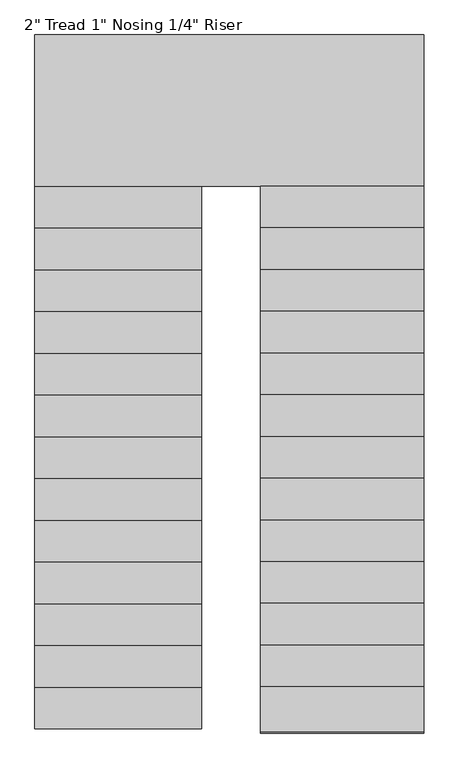
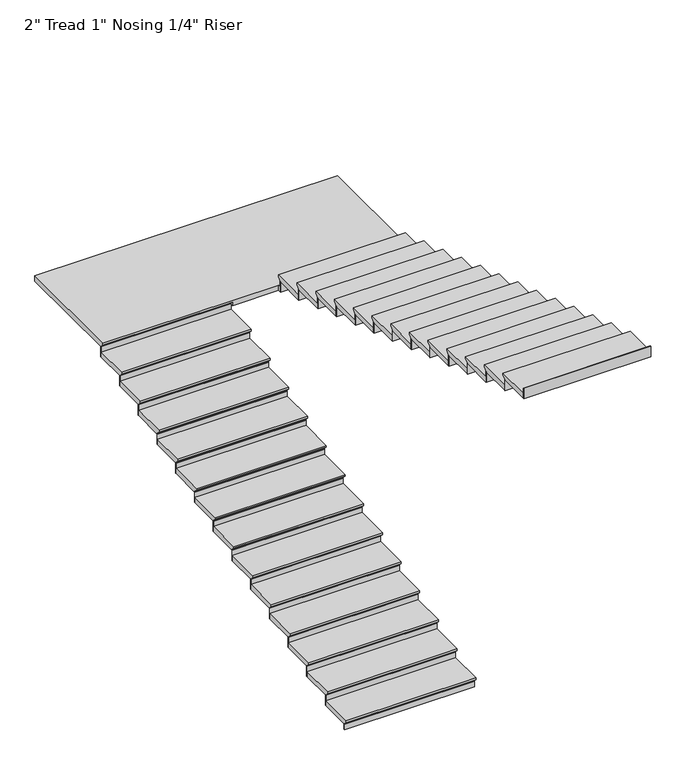
"""IFC4 building model written with IfcOpenShell, lengths in millimetres: stair flight geometry."""

from ifc_helpers import new_model, si_unit, origin, place, context, project, spatial, faceted_brep, source, transform, mapped, element, save


def stair_flight_ccf7fef2(model_context):
    return source(origin(), model_context, "Body", "Brep", [
        faceted_brep([(-629.5987998, 2564.5067329, 12885.9642857), (-629.5987998, 2564.5067329, 12905.0142857), (-1848.7987998, 2564.5067329, 12905.0142857), (-1848.7987998, 2564.5067329, 12885.9642857), (-629.5987998, 2589.9067329, 12860.5642857), (-1848.7987998, 2589.9067329, 12860.5642857), (-629.5987998, 2894.7067329, 12905.0142857), (-1848.7987998, 2894.7067329, 12905.0142857), (-1848.7987998, 2589.9067329, 12854.2142857), (-1848.7987998, 2894.7067329, 12854.2142857), (-629.5987998, 2894.7067329, 12854.2142857), (-629.5987998, 2589.9067329, 12854.2142857)], [[[0, 1, 2, 3]], [[4, 0, 3, 5]], [[2, 1, 6, 7]], [[8, 9, 10, 11]], [[2, 7, 9, 8, 5, 3]], [[8, 11, 4, 5]], [[6, 1, 0, 4, 11, 10]], [[7, 6, 10, 9]]]),
        faceted_brep([(-629.5987998, 2589.9067329, 12854.2142857), (-629.5987998, 2589.9067329, 12801.6), (-629.5987998, 2596.2567329, 12801.6), (-629.5987998, 2596.2567329, 12854.2142857), (-1848.7987998, 2589.9067329, 12854.2142857), (-1848.7987998, 2596.2567329, 12854.2142857), (-1848.7987998, 2596.2567329, 12801.6), (-1848.7987998, 2589.9067329, 12801.6)], [[[0, 1, 2, 3]], [[4, 5, 6, 7]], [[1, 0, 4, 7]], [[2, 1, 7, 6]], [[3, 2, 6, 5]], [[0, 3, 5, 4]]]),
        faceted_brep([(-629.5987998, 2894.7067329, 12957.6285714), (-629.5987998, 2894.7067329, 12854.2142857), (-629.5987998, 2901.0567329, 12854.2142857), (-629.5987998, 2901.0567329, 12957.6285714), (-1848.7987998, 2894.7067329, 12957.6285714), (-1848.7987998, 2901.0567329, 12957.6285714), (-1848.7987998, 2901.0567329, 12854.2142857), (-1848.7987998, 2894.7067329, 12854.2142857)], [[[0, 1, 2, 3]], [[4, 5, 6, 7]], [[1, 0, 4, 7]], [[2, 1, 7, 6]], [[3, 2, 6, 5]], [[0, 3, 5, 4]]]),
        faceted_brep([(-1848.7987998, 2869.3067329, 13008.4285714), (-629.5987998, 2869.3067329, 13008.4285714), (-629.5987998, 3199.5067329, 13008.4285714), (-1848.7987998, 3199.5067329, 13008.4285714), (-1848.7987998, 2894.7067329, 12957.6285714), (-1848.7987998, 3199.5067329, 12957.6285714), (-629.5987998, 3199.5067329, 12957.6285714), (-629.5987998, 2894.7067329, 12957.6285714), (-1848.7987998, 2894.7067329, 12963.9785714), (-1848.7987998, 2869.3067329, 12989.3785714), (-629.5987998, 2894.7067329, 12963.9785714), (-629.5987998, 2869.3067329, 12989.3785714)], [[[0, 1, 2, 3]], [[4, 5, 6, 7]], [[0, 3, 5, 4, 8, 9]], [[4, 7, 10, 8]], [[2, 1, 11, 10, 7, 6]], [[3, 2, 6, 5]], [[11, 1, 0, 9]], [[10, 11, 9, 8]]]),
        faceted_brep([(-629.5987998, 3199.5067329, 13061.0428571), (-629.5987998, 3199.5067329, 12957.6285714), (-629.5987998, 3205.8567329, 12957.6285714), (-629.5987998, 3205.8567329, 13061.0428571), (-1848.7987998, 3199.5067329, 13061.0428571), (-1848.7987998, 3205.8567329, 13061.0428571), (-1848.7987998, 3205.8567329, 12957.6285714), (-1848.7987998, 3199.5067329, 12957.6285714)], [[[0, 1, 2, 3]], [[4, 5, 6, 7]], [[1, 0, 4, 7]], [[2, 1, 7, 6]], [[3, 2, 6, 5]], [[0, 3, 5, 4]]]),
        faceted_brep([(-1848.7987998, 3174.1067329, 13111.8428571), (-629.5987998, 3174.1067329, 13111.8428571), (-629.5987998, 3504.3067329, 13111.8428571), (-1848.7987998, 3504.3067329, 13111.8428571), (-1848.7987998, 3199.5067329, 13061.0428571), (-1848.7987998, 3504.3067329, 13061.0428571), (-629.5987998, 3504.3067329, 13061.0428571), (-629.5987998, 3199.5067329, 13061.0428571), (-1848.7987998, 3199.5067329, 13067.3928571), (-1848.7987998, 3174.1067329, 13092.7928571), (-629.5987998, 3199.5067329, 13067.3928571), (-629.5987998, 3174.1067329, 13092.7928571)], [[[0, 1, 2, 3]], [[4, 5, 6, 7]], [[0, 3, 5, 4, 8, 9]], [[4, 7, 10, 8]], [[2, 1, 11, 10, 7, 6]], [[3, 2, 6, 5]], [[11, 1, 0, 9]], [[10, 11, 9, 8]]]),
        faceted_brep([(-629.5987998, 3504.3067329, 13164.4571429), (-629.5987998, 3504.3067329, 13061.0428571), (-629.5987998, 3510.6567329, 13061.0428571), (-629.5987998, 3510.6567329, 13164.4571429), (-1848.7987998, 3504.3067329, 13164.4571429), (-1848.7987998, 3510.6567329, 13164.4571429), (-1848.7987998, 3510.6567329, 13061.0428571), (-1848.7987998, 3504.3067329, 13061.0428571)], [[[0, 1, 2, 3]], [[4, 5, 6, 7]], [[1, 0, 4, 7]], [[2, 1, 7, 6]], [[3, 2, 6, 5]], [[0, 3, 5, 4]]]),
        faceted_brep([(-1848.7987998, 3478.9067329, 13215.2571429), (-629.5987998, 3478.9067329, 13215.2571429), (-629.5987998, 3809.1067329, 13215.2571429), (-1848.7987998, 3809.1067329, 13215.2571429), (-1848.7987998, 3504.3067329, 13164.4571429), (-1848.7987998, 3809.1067329, 13164.4571429), (-629.5987998, 3809.1067329, 13164.4571429), (-629.5987998, 3504.3067329, 13164.4571429), (-1848.7987998, 3504.3067329, 13170.8071429), (-1848.7987998, 3478.9067329, 13196.2071429), (-629.5987998, 3504.3067329, 13170.8071429), (-629.5987998, 3478.9067329, 13196.2071429)], [[[0, 1, 2, 3]], [[4, 5, 6, 7]], [[0, 3, 5, 4, 8, 9]], [[4, 7, 10, 8]], [[2, 1, 11, 10, 7, 6]], [[3, 2, 6, 5]], [[11, 1, 0, 9]], [[10, 11, 9, 8]]]),
        faceted_brep([(-629.5987998, 3809.1067329, 13267.8714286), (-629.5987998, 3809.1067329, 13164.4571429), (-629.5987998, 3815.4567329, 13164.4571429), (-629.5987998, 3815.4567329, 13267.8714286), (-1848.7987998, 3809.1067329, 13267.8714286), (-1848.7987998, 3815.4567329, 13267.8714286), (-1848.7987998, 3815.4567329, 13164.4571429), (-1848.7987998, 3809.1067329, 13164.4571429)], [[[0, 1, 2, 3]], [[4, 5, 6, 7]], [[1, 0, 4, 7]], [[2, 1, 7, 6]], [[3, 2, 6, 5]], [[0, 3, 5, 4]]]),
        faceted_brep([(-1848.7987998, 3783.7067329, 13318.6714286), (-629.5987998, 3783.7067329, 13318.6714286), (-629.5987998, 4113.9067329, 13318.6714286), (-1848.7987998, 4113.9067329, 13318.6714286), (-1848.7987998, 3809.1067329, 13267.8714286), (-1848.7987998, 4113.9067329, 13267.8714286), (-629.5987998, 4113.9067329, 13267.8714286), (-629.5987998, 3809.1067329, 13267.8714286), (-1848.7987998, 3809.1067329, 13274.2214286), (-1848.7987998, 3783.7067329, 13299.6214286), (-629.5987998, 3809.1067329, 13274.2214286), (-629.5987998, 3783.7067329, 13299.6214286)], [[[0, 1, 2, 3]], [[4, 5, 6, 7]], [[0, 3, 5, 4, 8, 9]], [[4, 7, 10, 8]], [[2, 1, 11, 10, 7, 6]], [[3, 2, 6, 5]], [[11, 1, 0, 9]], [[10, 11, 9, 8]]]),
        faceted_brep([(-629.5987998, 4113.9067329, 13371.2857143), (-629.5987998, 4113.9067329, 13267.8714286), (-629.5987998, 4120.2567329, 13267.8714286), (-629.5987998, 4120.2567329, 13371.2857143), (-1848.7987998, 4113.9067329, 13371.2857143), (-1848.7987998, 4120.2567329, 13371.2857143), (-1848.7987998, 4120.2567329, 13267.8714286), (-1848.7987998, 4113.9067329, 13267.8714286)], [[[0, 1, 2, 3]], [[4, 5, 6, 7]], [[1, 0, 4, 7]], [[2, 1, 7, 6]], [[3, 2, 6, 5]], [[0, 3, 5, 4]]]),
        faceted_brep([(-1848.7987998, 4088.5067329, 13422.0857143), (-629.5987998, 4088.5067329, 13422.0857143), (-629.5987998, 4418.7067329, 13422.0857143), (-1848.7987998, 4418.7067329, 13422.0857143), (-1848.7987998, 4113.9067329, 13371.2857143), (-1848.7987998, 4418.7067329, 13371.2857143), (-629.5987998, 4418.7067329, 13371.2857143), (-629.5987998, 4113.9067329, 13371.2857143), (-1848.7987998, 4113.9067329, 13377.6357143), (-1848.7987998, 4088.5067329, 13403.0357143), (-629.5987998, 4113.9067329, 13377.6357143), (-629.5987998, 4088.5067329, 13403.0357143)], [[[0, 1, 2, 3]], [[4, 5, 6, 7]], [[0, 3, 5, 4, 8, 9]], [[4, 7, 10, 8]], [[2, 1, 11, 10, 7, 6]], [[3, 2, 6, 5]], [[11, 1, 0, 9]], [[10, 11, 9, 8]]]),
        faceted_brep([(-629.5987998, 4418.7067329, 13474.7), (-629.5987998, 4418.7067329, 13371.2857143), (-629.5987998, 4425.0567329, 13371.2857143), (-629.5987998, 4425.0567329, 13474.7), (-1848.7987998, 4418.7067329, 13474.7), (-1848.7987998, 4425.0567329, 13474.7), (-1848.7987998, 4425.0567329, 13371.2857143), (-1848.7987998, 4418.7067329, 13371.2857143)], [[[0, 1, 2, 3]], [[4, 5, 6, 7]], [[1, 0, 4, 7]], [[2, 1, 7, 6]], [[3, 2, 6, 5]], [[0, 3, 5, 4]]]),
        faceted_brep([(-1848.7987998, 4393.3067329, 13525.5), (-629.5987998, 4393.3067329, 13525.5), (-629.5987998, 4723.5067329, 13525.5), (-1848.7987998, 4723.5067329, 13525.5), (-1848.7987998, 4418.7067329, 13474.7), (-1848.7987998, 4723.5067329, 13474.7), (-629.5987998, 4723.5067329, 13474.7), (-629.5987998, 4418.7067329, 13474.7), (-1848.7987998, 4418.7067329, 13481.05), (-1848.7987998, 4393.3067329, 13506.45), (-629.5987998, 4418.7067329, 13481.05), (-629.5987998, 4393.3067329, 13506.45)], [[[0, 1, 2, 3]], [[4, 5, 6, 7]], [[0, 3, 5, 4, 8, 9]], [[4, 7, 10, 8]], [[2, 1, 11, 10, 7, 6]], [[3, 2, 6, 5]], [[11, 1, 0, 9]], [[10, 11, 9, 8]]]),
        faceted_brep([(-629.5987998, 4723.5067329, 13578.1142857), (-629.5987998, 4723.5067329, 13474.7), (-629.5987998, 4729.8567329, 13474.7), (-629.5987998, 4729.8567329, 13578.1142857), (-1848.7987998, 4723.5067329, 13578.1142857), (-1848.7987998, 4729.8567329, 13578.1142857), (-1848.7987998, 4729.8567329, 13474.7), (-1848.7987998, 4723.5067329, 13474.7)], [[[0, 1, 2, 3]], [[4, 5, 6, 7]], [[1, 0, 4, 7]], [[2, 1, 7, 6]], [[3, 2, 6, 5]], [[0, 3, 5, 4]]]),
        faceted_brep([(-1848.7987998, 4698.1067329, 13628.9142857), (-629.5987998, 4698.1067329, 13628.9142857), (-629.5987998, 5028.3067329, 13628.9142857), (-1848.7987998, 5028.3067329, 13628.9142857), (-1848.7987998, 4723.5067329, 13578.1142857), (-1848.7987998, 5028.3067329, 13578.1142857), (-629.5987998, 5028.3067329, 13578.1142857), (-629.5987998, 4723.5067329, 13578.1142857), (-1848.7987998, 4723.5067329, 13584.4642857), (-1848.7987998, 4698.1067329, 13609.8642857), (-629.5987998, 4723.5067329, 13584.4642857), (-629.5987998, 4698.1067329, 13609.8642857)], [[[0, 1, 2, 3]], [[4, 5, 6, 7]], [[0, 3, 5, 4, 8, 9]], [[4, 7, 10, 8]], [[2, 1, 11, 10, 7, 6]], [[3, 2, 6, 5]], [[11, 1, 0, 9]], [[10, 11, 9, 8]]]),
        faceted_brep([(-629.5987998, 5028.3067329, 13681.5285714), (-629.5987998, 5028.3067329, 13578.1142857), (-629.5987998, 5034.6567329, 13578.1142857), (-629.5987998, 5034.6567329, 13681.5285714), (-1848.7987998, 5028.3067329, 13681.5285714), (-1848.7987998, 5034.6567329, 13681.5285714), (-1848.7987998, 5034.6567329, 13578.1142857), (-1848.7987998, 5028.3067329, 13578.1142857)], [[[0, 1, 2, 3]], [[4, 5, 6, 7]], [[1, 0, 4, 7]], [[2, 1, 7, 6]], [[3, 2, 6, 5]], [[0, 3, 5, 4]]]),
        faceted_brep([(-1848.7987998, 5002.9067329, 13732.3285714), (-629.5987998, 5002.9067329, 13732.3285714), (-629.5987998, 5333.1067329, 13732.3285714), (-1848.7987998, 5333.1067329, 13732.3285714), (-1848.7987998, 5028.3067329, 13681.5285714), (-1848.7987998, 5333.1067329, 13681.5285714), (-629.5987998, 5333.1067329, 13681.5285714), (-629.5987998, 5028.3067329, 13681.5285714), (-1848.7987998, 5028.3067329, 13687.8785714), (-1848.7987998, 5002.9067329, 13713.2785714), (-629.5987998, 5028.3067329, 13687.8785714), (-629.5987998, 5002.9067329, 13713.2785714)], [[[0, 1, 2, 3]], [[4, 5, 6, 7]], [[0, 3, 5, 4, 8, 9]], [[4, 7, 10, 8]], [[2, 1, 11, 10, 7, 6]], [[3, 2, 6, 5]], [[11, 1, 0, 9]], [[10, 11, 9, 8]]]),
        faceted_brep([(-629.5987998, 5333.1067329, 13784.9428571), (-629.5987998, 5333.1067329, 13681.5285714), (-629.5987998, 5339.4567329, 13681.5285714), (-629.5987998, 5339.4567329, 13784.9428571), (-1848.7987998, 5333.1067329, 13784.9428571), (-1848.7987998, 5339.4567329, 13784.9428571), (-1848.7987998, 5339.4567329, 13681.5285714), (-1848.7987998, 5333.1067329, 13681.5285714)], [[[0, 1, 2, 3]], [[4, 5, 6, 7]], [[1, 0, 4, 7]], [[2, 1, 7, 6]], [[3, 2, 6, 5]], [[0, 3, 5, 4]]]),
        faceted_brep([(-1848.7987998, 5307.7067329, 13835.7428571), (-629.5987998, 5307.7067329, 13835.7428571), (-629.5987998, 5637.9067329, 13835.7428571), (-1848.7987998, 5637.9067329, 13835.7428571), (-1848.7987998, 5333.1067329, 13784.9428571), (-1848.7987998, 5637.9067329, 13784.9428571), (-629.5987998, 5637.9067329, 13784.9428571), (-629.5987998, 5333.1067329, 13784.9428571), (-1848.7987998, 5333.1067329, 13791.2928571), (-1848.7987998, 5307.7067329, 13816.6928571), (-629.5987998, 5333.1067329, 13791.2928571), (-629.5987998, 5307.7067329, 13816.6928571)], [[[0, 1, 2, 3]], [[4, 5, 6, 7]], [[0, 3, 5, 4, 8, 9]], [[4, 7, 10, 8]], [[2, 1, 11, 10, 7, 6]], [[3, 2, 6, 5]], [[11, 1, 0, 9]], [[10, 11, 9, 8]]]),
        faceted_brep([(-629.5987998, 5637.9067329, 13888.3571429), (-629.5987998, 5637.9067329, 13784.9428571), (-629.5987998, 5644.2567329, 13784.9428571), (-629.5987998, 5644.2567329, 13888.3571429), (-1848.7987998, 5637.9067329, 13888.3571429), (-1848.7987998, 5644.2567329, 13888.3571429), (-1848.7987998, 5644.2567329, 13784.9428571), (-1848.7987998, 5637.9067329, 13784.9428571)], [[[0, 1, 2, 3]], [[4, 5, 6, 7]], [[1, 0, 4, 7]], [[2, 1, 7, 6]], [[3, 2, 6, 5]], [[0, 3, 5, 4]]]),
        faceted_brep([(-1848.7987998, 5612.5067329, 13939.1571429), (-629.5987998, 5612.5067329, 13939.1571429), (-629.5987998, 5942.7067329, 13939.1571429), (-1848.7987998, 5942.7067329, 13939.1571429), (-1848.7987998, 5637.9067329, 13888.3571429), (-1848.7987998, 5942.7067329, 13888.3571429), (-629.5987998, 5942.7067329, 13888.3571429), (-629.5987998, 5637.9067329, 13888.3571429), (-1848.7987998, 5637.9067329, 13894.7071429), (-1848.7987998, 5612.5067329, 13920.1071429), (-629.5987998, 5637.9067329, 13894.7071429), (-629.5987998, 5612.5067329, 13920.1071429)], [[[0, 1, 2, 3]], [[4, 5, 6, 7]], [[0, 3, 5, 4, 8, 9]], [[4, 7, 10, 8]], [[2, 1, 11, 10, 7, 6]], [[3, 2, 6, 5]], [[11, 1, 0, 9]], [[10, 11, 9, 8]]]),
        faceted_brep([(-629.5987998, 5942.7067329, 13991.7714286), (-629.5987998, 5942.7067329, 13888.3571429), (-629.5987998, 5949.0567329, 13888.3571429), (-629.5987998, 5949.0567329, 13991.7714286), (-1848.7987998, 5942.7067329, 13991.7714286), (-1848.7987998, 5949.0567329, 13991.7714286), (-1848.7987998, 5949.0567329, 13888.3571429), (-1848.7987998, 5942.7067329, 13888.3571429)], [[[0, 1, 2, 3]], [[4, 5, 6, 7]], [[1, 0, 4, 7]], [[2, 1, 7, 6]], [[3, 2, 6, 5]], [[0, 3, 5, 4]]]),
        faceted_brep([(-1848.7987998, 5917.3067329, 14042.5714286), (-629.5987998, 5917.3067329, 14042.5714286), (-629.5987998, 6247.5067329, 14042.5714286), (-1848.7987998, 6247.5067329, 14042.5714286), (-1848.7987998, 5942.7067329, 13991.7714286), (-1848.7987998, 6247.5067329, 13991.7714286), (-629.5987998, 6247.5067329, 13991.7714286), (-629.5987998, 5942.7067329, 13991.7714286), (-1848.7987998, 5942.7067329, 13998.1214286), (-1848.7987998, 5917.3067329, 14023.5214286), (-629.5987998, 5942.7067329, 13998.1214286), (-629.5987998, 5917.3067329, 14023.5214286)], [[[0, 1, 2, 3]], [[4, 5, 6, 7]], [[0, 3, 5, 4, 8, 9]], [[4, 7, 10, 8]], [[2, 1, 11, 10, 7, 6]], [[3, 2, 6, 5]], [[11, 1, 0, 9]], [[10, 11, 9, 8]]]),
        faceted_brep([(-629.5987998, 6247.5067329, 14095.1857143), (-629.5987998, 6247.5067329, 13991.7714286), (-629.5987998, 6253.8567329, 13991.7714286), (-629.5987998, 6253.8567329, 14095.1857143), (-1848.7987998, 6247.5067329, 14095.1857143), (-1848.7987998, 6253.8567329, 14095.1857143), (-1848.7987998, 6253.8567329, 13991.7714286), (-1848.7987998, 6247.5067329, 13991.7714286)], [[[0, 1, 2, 3]], [[4, 5, 6, 7]], [[1, 0, 4, 7]], [[2, 1, 7, 6]], [[3, 2, 6, 5]], [[0, 3, 5, 4]]]),
        faceted_brep([(-1848.7987998, 6222.1067329, 14145.9857143), (-629.5987998, 6222.1067329, 14145.9857143), (-629.5987998, 6552.3067329, 14145.9857143), (-1848.7987998, 6552.3067329, 14145.9857143), (-1848.7987998, 6247.5067329, 14095.1857143), (-1848.7987998, 6552.3067329, 14095.1857143), (-629.5987998, 6552.3067329, 14095.1857143), (-629.5987998, 6247.5067329, 14095.1857143), (-1848.7987998, 6247.5067329, 14101.5357143), (-1848.7987998, 6222.1067329, 14126.9357143), (-629.5987998, 6247.5067329, 14101.5357143), (-629.5987998, 6222.1067329, 14126.9357143)], [[[0, 1, 2, 3]], [[4, 5, 6, 7]], [[0, 3, 5, 4, 8, 9]], [[4, 7, 10, 8]], [[2, 1, 11, 10, 7, 6]], [[3, 2, 6, 5]], [[11, 1, 0, 9]], [[10, 11, 9, 8]]]),
        faceted_brep([(-629.5987998, 6552.3067329, 14198.6), (-629.5987998, 6552.3067329, 14095.1857143), (-629.5987998, 6558.6567329, 14095.1857143), (-629.5987998, 6558.6567329, 14198.6), (-1848.7987998, 6552.3067329, 14198.6), (-1848.7987998, 6558.6567329, 14198.6), (-1848.7987998, 6558.6567329, 14095.1857143), (-1848.7987998, 6552.3067329, 14095.1857143)], [[[0, 1, 2, 3]], [[4, 5, 6, 7]], [[1, 0, 4, 7]], [[2, 1, 7, 6]], [[3, 2, 6, 5]], [[0, 3, 5, 4]]]),
        faceted_brep([(996.0012002, 6501.5067329, 14249.4), (996.0012002, 7631.8067329, 14249.4), (-1848.7987998, 7631.8067329, 14249.4), (-1848.7987998, 6526.9067329, 14249.4), (-197.7987915, 6526.9067329, 14249.4), (-197.7987915, 6501.5067329, 14249.4), (996.0012002, 7631.8067329, 14198.6), (996.0012002, 6501.5067329, 14198.6), (-197.7987915, 6501.5067329, 14198.6), (-197.7987915, 6526.9067329, 14198.6), (-629.5987998, 6526.9067329, 14198.6), (-629.5987998, 6552.3067329, 14198.6), (-1848.7987998, 6552.3067329, 14198.6), (-1848.7987998, 7631.8067329, 14198.6), (-629.5987998, 6552.3067329, 14204.95), (-1848.7987998, 6552.3067329, 14204.95), (-1848.7987998, 6526.9067329, 14230.35), (-629.5987998, 6526.9067329, 14230.35)], [[[0, 1, 2, 3, 4, 5]], [[6, 7, 8, 9, 10, 11, 12, 13]], [[1, 0, 7, 6]], [[2, 1, 6, 13]], [[12, 11, 14, 15]], [[4, 3, 16, 17, 10, 9]], [[5, 4, 9, 8]], [[0, 5, 8, 7]], [[16, 15, 14, 17]], [[3, 2, 13, 12, 15, 16]], [[11, 10, 17, 14]]]),
        faceted_brep([(-197.7987915, 6501.5067329, 14302.0142857), (-197.7987915, 6501.5067329, 14198.6), (-197.7987915, 6495.1567329, 14198.6), (-197.7987915, 6495.1567329, 14302.0142857), (996.0012002, 6501.5067329, 14302.0142857), (996.0012002, 6495.1567329, 14302.0142857), (996.0012002, 6495.1567329, 14198.6), (996.0012002, 6501.5067329, 14198.6)], [[[0, 1, 2, 3]], [[4, 5, 6, 7]], [[1, 0, 4, 7]], [[2, 1, 7, 6]], [[3, 2, 6, 5]], [[0, 3, 5, 4]]]),
        faceted_brep([(996.0012002, 6526.9067329, 14352.8142857), (-197.7987915, 6526.9067329, 14352.8142857), (-197.7987915, 6196.7067329, 14352.8142857), (996.0012002, 6196.7067329, 14352.8142857), (996.0012002, 6501.5067329, 14302.0142857), (996.0012002, 6196.7067329, 14302.0142857), (-197.7987915, 6196.7067329, 14302.0142857), (-197.7987915, 6501.5067329, 14302.0142857), (996.0012002, 6501.5067329, 14308.3642857), (996.0012002, 6526.9067329, 14333.7642857), (-197.7987915, 6501.5067329, 14308.3642857), (-197.7987915, 6526.9067329, 14333.7642857)], [[[0, 1, 2, 3]], [[4, 5, 6, 7]], [[0, 3, 5, 4, 8, 9]], [[4, 7, 10, 8]], [[2, 1, 11, 10, 7, 6]], [[3, 2, 6, 5]], [[11, 1, 0, 9]], [[10, 11, 9, 8]]]),
        faceted_brep([(-197.7987915, 6196.7067329, 14405.4285714), (-197.7987915, 6196.7067329, 14302.0142857), (-197.7987915, 6190.3567329, 14302.0142857), (-197.7987915, 6190.3567329, 14405.4285714), (996.0012002, 6196.7067329, 14405.4285714), (996.0012002, 6190.3567329, 14405.4285714), (996.0012002, 6190.3567329, 14302.0142857), (996.0012002, 6196.7067329, 14302.0142857)], [[[0, 1, 2, 3]], [[4, 5, 6, 7]], [[1, 0, 4, 7]], [[2, 1, 7, 6]], [[3, 2, 6, 5]], [[0, 3, 5, 4]]]),
        faceted_brep([(996.0012002, 6222.1067329, 14456.2285714), (-197.7987915, 6222.1067329, 14456.2285714), (-197.7987915, 5891.9067329, 14456.2285714), (996.0012002, 5891.9067329, 14456.2285714), (996.0012002, 6196.7067329, 14405.4285714), (996.0012002, 5891.9067329, 14405.4285714), (-197.7987915, 5891.9067329, 14405.4285714), (-197.7987915, 6196.7067329, 14405.4285714), (996.0012002, 6196.7067329, 14411.7785714), (996.0012002, 6222.1067329, 14437.1785714), (-197.7987915, 6196.7067329, 14411.7785714), (-197.7987915, 6222.1067329, 14437.1785714)], [[[0, 1, 2, 3]], [[4, 5, 6, 7]], [[0, 3, 5, 4, 8, 9]], [[4, 7, 10, 8]], [[2, 1, 11, 10, 7, 6]], [[3, 2, 6, 5]], [[11, 1, 0, 9]], [[10, 11, 9, 8]]]),
        faceted_brep([(-197.7987915, 5891.9067329, 14508.8428571), (-197.7987915, 5891.9067329, 14405.4285714), (-197.7987915, 5885.5567329, 14405.4285714), (-197.7987915, 5885.5567329, 14508.8428571), (996.0012002, 5891.9067329, 14508.8428571), (996.0012002, 5885.5567329, 14508.8428571), (996.0012002, 5885.5567329, 14405.4285714), (996.0012002, 5891.9067329, 14405.4285714)], [[[0, 1, 2, 3]], [[4, 5, 6, 7]], [[1, 0, 4, 7]], [[2, 1, 7, 6]], [[3, 2, 6, 5]], [[0, 3, 5, 4]]]),
        faceted_brep([(996.0012002, 5917.3067329, 14559.6428571), (-197.7987915, 5917.3067329, 14559.6428571), (-197.7987915, 5587.1067329, 14559.6428571), (996.0012002, 5587.1067329, 14559.6428571), (996.0012002, 5891.9067329, 14508.8428571), (996.0012002, 5587.1067329, 14508.8428571), (-197.7987915, 5587.1067329, 14508.8428571), (-197.7987915, 5891.9067329, 14508.8428571), (996.0012002, 5891.9067329, 14515.1928571), (996.0012002, 5917.3067329, 14540.5928571), (-197.7987915, 5891.9067329, 14515.1928571), (-197.7987915, 5917.3067329, 14540.5928571)], [[[0, 1, 2, 3]], [[4, 5, 6, 7]], [[0, 3, 5, 4, 8, 9]], [[4, 7, 10, 8]], [[2, 1, 11, 10, 7, 6]], [[3, 2, 6, 5]], [[11, 1, 0, 9]], [[10, 11, 9, 8]]]),
        faceted_brep([(-197.7987915, 5587.1067329, 14612.2571429), (-197.7987915, 5587.1067329, 14508.8428571), (-197.7987915, 5580.7567329, 14508.8428571), (-197.7987915, 5580.7567329, 14612.2571429), (996.0012002, 5587.1067329, 14612.2571429), (996.0012002, 5580.7567329, 14612.2571429), (996.0012002, 5580.7567329, 14508.8428571), (996.0012002, 5587.1067329, 14508.8428571)], [[[0, 1, 2, 3]], [[4, 5, 6, 7]], [[1, 0, 4, 7]], [[2, 1, 7, 6]], [[3, 2, 6, 5]], [[0, 3, 5, 4]]]),
        faceted_brep([(996.0012002, 5612.5067329, 14663.0571429), (-197.7987915, 5612.5067329, 14663.0571429), (-197.7987915, 5282.3067329, 14663.0571429), (996.0012002, 5282.3067329, 14663.0571429), (996.0012002, 5587.1067329, 14612.2571429), (996.0012002, 5282.3067329, 14612.2571429), (-197.7987915, 5282.3067329, 14612.2571429), (-197.7987915, 5587.1067329, 14612.2571429), (996.0012002, 5587.1067329, 14618.6071429), (996.0012002, 5612.5067329, 14644.0071429), (-197.7987915, 5587.1067329, 14618.6071429), (-197.7987915, 5612.5067329, 14644.0071429)], [[[0, 1, 2, 3]], [[4, 5, 6, 7]], [[0, 3, 5, 4, 8, 9]], [[4, 7, 10, 8]], [[2, 1, 11, 10, 7, 6]], [[3, 2, 6, 5]], [[11, 1, 0, 9]], [[10, 11, 9, 8]]]),
        faceted_brep([(-197.7987915, 5282.3067329, 14715.6714286), (-197.7987915, 5282.3067329, 14612.2571429), (-197.7987915, 5275.9567329, 14612.2571429), (-197.7987915, 5275.9567329, 14715.6714286), (996.0012002, 5282.3067329, 14715.6714286), (996.0012002, 5275.9567329, 14715.6714286), (996.0012002, 5275.9567329, 14612.2571429), (996.0012002, 5282.3067329, 14612.2571429)], [[[0, 1, 2, 3]], [[4, 5, 6, 7]], [[1, 0, 4, 7]], [[2, 1, 7, 6]], [[3, 2, 6, 5]], [[0, 3, 5, 4]]]),
        faceted_brep([(996.0012002, 5307.7067329, 14766.4714286), (-197.7987915, 5307.7067329, 14766.4714286), (-197.7987915, 4977.5067329, 14766.4714286), (996.0012002, 4977.5067329, 14766.4714286), (996.0012002, 5282.3067329, 14715.6714286), (996.0012002, 4977.5067329, 14715.6714286), (-197.7987915, 4977.5067329, 14715.6714286), (-197.7987915, 5282.3067329, 14715.6714286), (996.0012002, 5282.3067329, 14722.0214286), (996.0012002, 5307.7067329, 14747.4214286), (-197.7987915, 5282.3067329, 14722.0214286), (-197.7987915, 5307.7067329, 14747.4214286)], [[[0, 1, 2, 3]], [[4, 5, 6, 7]], [[0, 3, 5, 4, 8, 9]], [[4, 7, 10, 8]], [[2, 1, 11, 10, 7, 6]], [[3, 2, 6, 5]], [[11, 1, 0, 9]], [[10, 11, 9, 8]]]),
        faceted_brep([(-197.7987915, 4977.5067329, 14819.0857143), (-197.7987915, 4977.5067329, 14715.6714286), (-197.7987915, 4971.1567329, 14715.6714286), (-197.7987915, 4971.1567329, 14819.0857143), (996.0012002, 4977.5067329, 14819.0857143), (996.0012002, 4971.1567329, 14819.0857143), (996.0012002, 4971.1567329, 14715.6714286), (996.0012002, 4977.5067329, 14715.6714286)], [[[0, 1, 2, 3]], [[4, 5, 6, 7]], [[1, 0, 4, 7]], [[2, 1, 7, 6]], [[3, 2, 6, 5]], [[0, 3, 5, 4]]]),
        faceted_brep([(996.0012002, 5002.9067329, 14869.8857143), (-197.7987915, 5002.9067329, 14869.8857143), (-197.7987915, 4672.7067329, 14869.8857143), (996.0012002, 4672.7067329, 14869.8857143), (996.0012002, 4977.5067329, 14819.0857143), (996.0012002, 4672.7067329, 14819.0857143), (-197.7987915, 4672.7067329, 14819.0857143), (-197.7987915, 4977.5067329, 14819.0857143), (996.0012002, 4977.5067329, 14825.4357143), (996.0012002, 5002.9067329, 14850.8357143), (-197.7987915, 4977.5067329, 14825.4357143), (-197.7987915, 5002.9067329, 14850.8357143)], [[[0, 1, 2, 3]], [[4, 5, 6, 7]], [[0, 3, 5, 4, 8, 9]], [[4, 7, 10, 8]], [[2, 1, 11, 10, 7, 6]], [[3, 2, 6, 5]], [[11, 1, 0, 9]], [[10, 11, 9, 8]]]),
        faceted_brep([(-197.7987915, 4672.7067329, 14922.5), (-197.7987915, 4672.7067329, 14819.0857143), (-197.7987915, 4666.3567329, 14819.0857143), (-197.7987915, 4666.3567329, 14922.5), (996.0012002, 4672.7067329, 14922.5), (996.0012002, 4666.3567329, 14922.5), (996.0012002, 4666.3567329, 14819.0857143), (996.0012002, 4672.7067329, 14819.0857143)], [[[0, 1, 2, 3]], [[4, 5, 6, 7]], [[1, 0, 4, 7]], [[2, 1, 7, 6]], [[3, 2, 6, 5]], [[0, 3, 5, 4]]]),
        faceted_brep([(996.0012002, 4698.1067329, 14973.3), (-197.7987915, 4698.1067329, 14973.3), (-197.7987915, 4367.9067329, 14973.3), (996.0012002, 4367.9067329, 14973.3), (996.0012002, 4672.7067329, 14922.5), (996.0012002, 4367.9067329, 14922.5), (-197.7987915, 4367.9067329, 14922.5), (-197.7987915, 4672.7067329, 14922.5), (996.0012002, 4672.7067329, 14928.85), (996.0012002, 4698.1067329, 14954.25), (-197.7987915, 4672.7067329, 14928.85), (-197.7987915, 4698.1067329, 14954.25)], [[[0, 1, 2, 3]], [[4, 5, 6, 7]], [[0, 3, 5, 4, 8, 9]], [[4, 7, 10, 8]], [[2, 1, 11, 10, 7, 6]], [[3, 2, 6, 5]], [[11, 1, 0, 9]], [[10, 11, 9, 8]]]),
        faceted_brep([(-197.7987915, 4367.9067329, 15025.9142857), (-197.7987915, 4367.9067329, 14922.5), (-197.7987915, 4361.5567329, 14922.5), (-197.7987915, 4361.5567329, 15025.9142857), (996.0012002, 4367.9067329, 15025.9142857), (996.0012002, 4361.5567329, 15025.9142857), (996.0012002, 4361.5567329, 14922.5), (996.0012002, 4367.9067329, 14922.5)], [[[0, 1, 2, 3]], [[4, 5, 6, 7]], [[1, 0, 4, 7]], [[2, 1, 7, 6]], [[3, 2, 6, 5]], [[0, 3, 5, 4]]]),
        faceted_brep([(996.0012002, 4393.3067329, 15076.7142857), (-197.7987915, 4393.3067329, 15076.7142857), (-197.7987915, 4063.1067329, 15076.7142857), (996.0012002, 4063.1067329, 15076.7142857), (996.0012002, 4367.9067329, 15025.9142857), (996.0012002, 4063.1067329, 15025.9142857), (-197.7987915, 4063.1067329, 15025.9142857), (-197.7987915, 4367.9067329, 15025.9142857), (996.0012002, 4367.9067329, 15032.2642857), (996.0012002, 4393.3067329, 15057.6642857), (-197.7987915, 4367.9067329, 15032.2642857), (-197.7987915, 4393.3067329, 15057.6642857)], [[[0, 1, 2, 3]], [[4, 5, 6, 7]], [[0, 3, 5, 4, 8, 9]], [[4, 7, 10, 8]], [[2, 1, 11, 10, 7, 6]], [[3, 2, 6, 5]], [[11, 1, 0, 9]], [[10, 11, 9, 8]]]),
        faceted_brep([(-197.7987915, 4063.1067329, 15129.3285714), (-197.7987915, 4063.1067329, 15025.9142857), (-197.7987915, 4056.7567329, 15025.9142857), (-197.7987915, 4056.7567329, 15129.3285714), (996.0012002, 4063.1067329, 15129.3285714), (996.0012002, 4056.7567329, 15129.3285714), (996.0012002, 4056.7567329, 15025.9142857), (996.0012002, 4063.1067329, 15025.9142857)], [[[0, 1, 2, 3]], [[4, 5, 6, 7]], [[1, 0, 4, 7]], [[2, 1, 7, 6]], [[3, 2, 6, 5]], [[0, 3, 5, 4]]]),
        faceted_brep([(996.0012002, 4088.5067329, 15180.1285714), (-197.7987915, 4088.5067329, 15180.1285714), (-197.7987915, 3758.3067329, 15180.1285714), (996.0012002, 3758.3067329, 15180.1285714), (996.0012002, 4063.1067329, 15129.3285714), (996.0012002, 3758.3067329, 15129.3285714), (-197.7987915, 3758.3067329, 15129.3285714), (-197.7987915, 4063.1067329, 15129.3285714), (996.0012002, 4063.1067329, 15135.6785714), (996.0012002, 4088.5067329, 15161.0785714), (-197.7987915, 4063.1067329, 15135.6785714), (-197.7987915, 4088.5067329, 15161.0785714)], [[[0, 1, 2, 3]], [[4, 5, 6, 7]], [[0, 3, 5, 4, 8, 9]], [[4, 7, 10, 8]], [[2, 1, 11, 10, 7, 6]], [[3, 2, 6, 5]], [[11, 1, 0, 9]], [[10, 11, 9, 8]]]),
        faceted_brep([(-197.7987915, 3758.3067329, 15232.7428571), (-197.7987915, 3758.3067329, 15129.3285714), (-197.7987915, 3751.9567329, 15129.3285714), (-197.7987915, 3751.9567329, 15232.7428571), (996.0012002, 3758.3067329, 15232.7428571), (996.0012002, 3751.9567329, 15232.7428571), (996.0012002, 3751.9567329, 15129.3285714), (996.0012002, 3758.3067329, 15129.3285714)], [[[0, 1, 2, 3]], [[4, 5, 6, 7]], [[1, 0, 4, 7]], [[2, 1, 7, 6]], [[3, 2, 6, 5]], [[0, 3, 5, 4]]]),
        faceted_brep([(996.0012002, 3783.7067329, 15283.5428571), (-197.7987915, 3783.7067329, 15283.5428571), (-197.7987915, 3453.5067329, 15283.5428571), (996.0012002, 3453.5067329, 15283.5428571), (996.0012002, 3758.3067329, 15232.7428571), (996.0012002, 3453.5067329, 15232.7428571), (-197.7987915, 3453.5067329, 15232.7428571), (-197.7987915, 3758.3067329, 15232.7428571), (996.0012002, 3758.3067329, 15239.0928571), (996.0012002, 3783.7067329, 15264.4928571), (-197.7987915, 3758.3067329, 15239.0928571), (-197.7987915, 3783.7067329, 15264.4928571)], [[[0, 1, 2, 3]], [[4, 5, 6, 7]], [[0, 3, 5, 4, 8, 9]], [[4, 7, 10, 8]], [[2, 1, 11, 10, 7, 6]], [[3, 2, 6, 5]], [[11, 1, 0, 9]], [[10, 11, 9, 8]]]),
        faceted_brep([(-197.7987915, 3453.5067329, 15336.1571429), (-197.7987915, 3453.5067329, 15232.7428571), (-197.7987915, 3447.1567329, 15232.7428571), (-197.7987915, 3447.1567329, 15336.1571429), (996.0012002, 3453.5067329, 15336.1571429), (996.0012002, 3447.1567329, 15336.1571429), (996.0012002, 3447.1567329, 15232.7428571), (996.0012002, 3453.5067329, 15232.7428571)], [[[0, 1, 2, 3]], [[4, 5, 6, 7]], [[1, 0, 4, 7]], [[2, 1, 7, 6]], [[3, 2, 6, 5]], [[0, 3, 5, 4]]]),
        faceted_brep([(996.0012002, 3478.9067329, 15386.9571429), (-197.7987915, 3478.9067329, 15386.9571429), (-197.7987915, 3148.7067329, 15386.9571429), (996.0012002, 3148.7067329, 15386.9571429), (996.0012002, 3453.5067329, 15336.1571429), (996.0012002, 3148.7067329, 15336.1571429), (-197.7987915, 3148.7067329, 15336.1571429), (-197.7987915, 3453.5067329, 15336.1571429), (996.0012002, 3453.5067329, 15342.5071429), (996.0012002, 3478.9067329, 15367.9071429), (-197.7987915, 3453.5067329, 15342.5071429), (-197.7987915, 3478.9067329, 15367.9071429)], [[[0, 1, 2, 3]], [[4, 5, 6, 7]], [[0, 3, 5, 4, 8, 9]], [[4, 7, 10, 8]], [[2, 1, 11, 10, 7, 6]], [[3, 2, 6, 5]], [[11, 1, 0, 9]], [[10, 11, 9, 8]]]),
        faceted_brep([(-197.7987915, 3148.7067329, 15439.5714286), (-197.7987915, 3148.7067329, 15336.1571429), (-197.7987915, 3142.3567329, 15336.1571429), (-197.7987915, 3142.3567329, 15439.5714286), (996.0012002, 3148.7067329, 15439.5714286), (996.0012002, 3142.3567329, 15439.5714286), (996.0012002, 3142.3567329, 15336.1571429), (996.0012002, 3148.7067329, 15336.1571429)], [[[0, 1, 2, 3]], [[4, 5, 6, 7]], [[1, 0, 4, 7]], [[2, 1, 7, 6]], [[3, 2, 6, 5]], [[0, 3, 5, 4]]]),
        faceted_brep([(996.0012002, 3174.1067329, 15490.3714286), (-197.7987915, 3174.1067329, 15490.3714286), (-197.7987915, 2843.9067329, 15490.3714286), (996.0012002, 2843.9067329, 15490.3714286), (996.0012002, 3148.7067329, 15439.5714286), (996.0012002, 2843.9067329, 15439.5714286), (-197.7987915, 2843.9067329, 15439.5714286), (-197.7987915, 3148.7067329, 15439.5714286), (996.0012002, 3148.7067329, 15445.9214286), (996.0012002, 3174.1067329, 15471.3214286), (-197.7987915, 3148.7067329, 15445.9214286), (-197.7987915, 3174.1067329, 15471.3214286)], [[[0, 1, 2, 3]], [[4, 5, 6, 7]], [[0, 3, 5, 4, 8, 9]], [[4, 7, 10, 8]], [[2, 1, 11, 10, 7, 6]], [[3, 2, 6, 5]], [[11, 1, 0, 9]], [[10, 11, 9, 8]]]),
        faceted_brep([(-197.7987915, 2843.9067329, 15542.9857143), (-197.7987915, 2843.9067329, 15439.5714286), (-197.7987915, 2837.5567329, 15439.5714286), (-197.7987915, 2837.5567329, 15542.9857143), (996.0012002, 2843.9067329, 15542.9857143), (996.0012002, 2837.5567329, 15542.9857143), (996.0012002, 2837.5567329, 15439.5714286), (996.0012002, 2843.9067329, 15439.5714286)], [[[0, 1, 2, 3]], [[4, 5, 6, 7]], [[1, 0, 4, 7]], [[2, 1, 7, 6]], [[3, 2, 6, 5]], [[0, 3, 5, 4]]]),
        faceted_brep([(-197.7987915, 2539.1067329, 15646.4), (-197.7987915, 2539.1067329, 15542.9857143), (-197.7987915, 2532.7567329, 15542.9857143), (-197.7987915, 2532.7567329, 15646.4), (996.0012002, 2539.1067329, 15646.4), (996.0012002, 2532.7567329, 15646.4), (996.0012002, 2532.7567329, 15542.9857143), (996.0012002, 2539.1067329, 15542.9857143)], [[[0, 1, 2, 3]], [[4, 5, 6, 7]], [[1, 0, 4, 7]], [[2, 1, 7, 6]], [[3, 2, 6, 5]], [[0, 3, 5, 4]]]),
        faceted_brep([(996.0012002, 2869.3067329, 15593.7857143), (-197.7987915, 2869.3067329, 15593.7857143), (-197.7987915, 2539.1067329, 15593.7857143), (996.0012002, 2539.1067329, 15593.7857143), (996.0012002, 2843.9067329, 15542.9857143), (996.0012002, 2539.1067329, 15542.9857143), (-197.7987915, 2539.1067329, 15542.9857143), (-197.7987915, 2843.9067329, 15542.9857143), (996.0012002, 2843.9067329, 15549.3357143), (996.0012002, 2869.3067329, 15574.7357143), (-197.7987915, 2843.9067329, 15549.3357143), (-197.7987915, 2869.3067329, 15574.7357143)], [[[0, 1, 2, 3]], [[4, 5, 6, 7]], [[0, 3, 5, 4, 8, 9]], [[4, 7, 10, 8]], [[2, 1, 11, 10, 7, 6]], [[3, 2, 6, 5]], [[11, 1, 0, 9]], [[10, 11, 9, 8]]]),
    ])


if __name__ == "__main__":
    model = new_model("IFC4")
    model_context = context("Model", 3, world=origin())
    ifc_project = project(units=[si_unit("LENGTHUNIT", "METRE", prefix="MILLI")], contexts=[model_context])
    site = spatial("IfcSite", under=ifc_project)
    building = spatial("IfcBuilding", under=site)
    placement = place(None, origin())
    stair_flight_shape = stair_flight_ccf7fef2(model_context)
    element("IfcStairFlight", 1, ObjectType="2\" Tread 1\" Nosing 1/4\" Riser", at=placement, inside=building, context=model_context, shape_type="MappedRepresentation", body=[
        mapped(stair_flight_shape, transform((0.0, 0.0, 0.0), x_axis=(1.0, 0.0, 0.0), y_axis=(0.0, 1.0, 0.0), z_axis=(0.0, 0.0, 1.0))),
    ])
    save(model, "model.ifc")
